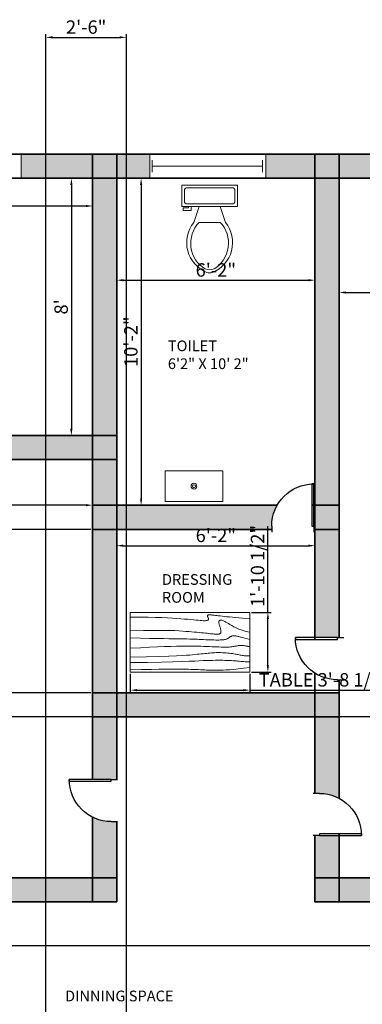
# Model space of a CAD drawing. Units: millimetres. Extents: x 2936 to 3516, y 349 to 1320.
# Tile 4 of 5: x 3187 to 3315, y 948 to 1315. Entities that reach past the tile are written whole.
import ezdxf

# ---------------------------------------------------------------- set-up
doc = ezdxf.new("R2010")
doc.units = ezdxf.units.MM
for name, color, linetype, lineweight in [('A-ANNO-DIMS', 3, 'Continuous', 13), ('A-AREA-IDEN', 190, 'Continuous', 18), ('A-FLOR-FIXT', 140, 'Continuous', 18), ('A-WALL-PATT', 50, 'Continuous', 13), ('doors', 10, 'Continuous', 25), ('furniture', 140, 'Continuous', 18), ('walls', 50, 'Continuous', 35), ('windows', 30, 'Continuous', 18)]:
    doc.layers.add(name, color=color, linetype=linetype, lineweight=lineweight)
doc.styles.get("Standard").update_dxf_attribs({"font": 'arial.ttf'})
doc.dimstyles.new('ISO-25', dxfattribs={"dimtxt": 5, "dimasz": 2.5, "dimexe": 1.25, "dimexo": 0.625, "dimtad": 1, "dimdec": 0, "dimlunit": 3, "dimtxsty": 'Standard', "dimcen": 2.5, "dimadec": 0, "dimazin": 0, "dimtfac": 1, "dimtdec": 0, "dimtmove": 0, "dimatfit": 3, "dimfxl": 1, "dimarcsym": 0})

# ---------------------------------------------------------------- blocks, each defined once
blk = doc.blocks.new('*U2')
for p, q in [((0, 0), (0, -6)), ((40, 0), (40, -6))]:
    blk.add_line(p, q)
blk.add_lwpolyline([(0, 0), (0, 40), (1.75, 40), (1.75, 0)], close=True)
blk.add_arc((0, 0), 40, 0, 90)
blk = doc.blocks.new('*U4')
for p, q in [((0, 4), (0, 0)), ((36, 4), (36, 0)), ((0, 2), (36, 2))]:
    blk.add_line(p, q)
blk = doc.blocks.new('Toilet - top')
for p, q in [((9.5, -6), (9.5, -2)), ((-10, -8.5), (-8, -8.5)), ((-10, -9.5), (-10, -8.5)), ((-7, -9.5), (-10, -9.5)), ((-8, -8.5), (-8, -8)), ((-7, -8), (-7, -9.5)), ((-4, -8), (-6, -14)), ((4, -8), (6, -14)), ((4, -14), (-4, -14))]:
    blk.add_line(p, q)
blk.add_lwpolyline([(10.5, -8), (10.5, 0), (-10.5, 0), (-10.5, -8)], close=True)
for points in [[(-9.5, -2), (-9.5, -6)], [(8.5, -1), (-8.5, -1)], [(-8.5, -7), (8.5, -7)]]:
    blk.add_lwpolyline(points)
for centre, radius, start, end in [((-8.62, -1.88), 0.884, 81.8699, 188.1301), ((8.62, -1.88), 0.884, 351.8699, 98.1301), ((-8.62, -6.12), 0.884, 171.8699, 278.1301), ((8.62, -6.12), 0.884, 261.8699, 8.1301), ((3.52, -21.58), 12.17, 141.4691, 247.9714), ((4.2, -21.82), 11.33, 136.3677, 238.9468), ((-3.52, -21.58), 12.17, 292.0284, 38.5307), ((-4.2, -21.82), 11.33, 301.053, 43.6321), ((0, -27.88), 4, 245.7318, 294.2682), ((0, -29), 4, 254.8605, 285.1395)]:
    blk.add_arc(centre, radius, start, end)
blk = doc.blocks.new('Table - Rectangular Woodgrain 60 x 30 in.')
for p, q in [((0, 0), (0, -30)), ((60, 0), (0, 0)), ((60, -30), (60, 0)), ((0, -30), (60, -30))]:
    blk.add_line(p, q)
for points in [[(0, -2.4), (4.8155, -2.418), (9.0302, -2.4688), (12.709, -2.5477), (15.9167, -2.65), (18.7181, -2.7711), (21.1781, -2.9063), (23.3616, -3.0508), (25.3333, -3.2), (27.1477, -3.3495), (28.8172, -3.4958), (30.3437, -3.636), (31.7291, -3.7667), (32.9756, -3.8849), (34.0849, -3.9875), (35.059, -4.0714), (35.9, -4.1334), (36.6114, -4.1711), (37.2041, -4.1854), (37.6906, -4.1779), (38.0833, -4.15), (38.3948, -4.1034), (38.6375, -4.0396), (38.8239, -3.9602), (38.9666, -3.8667), (39.0764, -3.7608), (39.1573, -3.6448), (39.2116, -3.521), (39.2416, -3.3917), (39.2498, -3.2593), (39.2385, -3.1261), (39.21, -2.9944), (39.1666, -2.8667), (39.111, -2.7447), (39.0468, -2.6281), (38.978, -2.5163), (38.9083, -2.4083), (38.8418, -2.3035), (38.7823, -2.201), (38.7337, -2.1001), (38.7, -2), (38.6844, -1.9003), (38.6875, -1.8021), (38.7094, -1.707), (38.75, -1.6167), (38.8094, -1.5326), (38.8875, -1.4563), (38.9844, -1.3893), (39.1, -1.3333), (39.2351, -1.2896), (39.3937, -1.2583), (39.5804, -1.2396), (39.8, -1.2333), (40.057, -1.2396), (40.3562, -1.2583), (40.7023, -1.2896), (41.1, -1.3333), (41.5547, -1.3895), (42.0755, -1.4573), (42.6721, -1.5361), (43.3542, -1.625), (44.1316, -1.7233), (45.014, -1.8302), (46.0114, -1.9449), (47.1333, -2.0667), (48.3862, -2.1947), (49.7625, -2.3281), (51.2513, -2.4663), (52.8416, -2.6083), (54.5226, -2.7535), (56.2833, -2.9011), (58.1127, -3.0501), (60, -3.2)], [(0, -9.2), (6.5759, -9.0858), (11.9385, -9.0365), (16.2527, -9.0418), (19.6833, -9.0917), (22.3952, -9.1759), (24.5531, -9.2844), (26.322, -9.4069), (27.8666, -9.5333), (29.3241, -9.6553), (30.7203, -9.7719), (32.0532, -9.8837), (33.3208, -9.9917), (34.5213, -10.0965), (35.6526, -10.199), (36.7128, -10.2999), (37.7, -10.4), (38.6129, -10.4996), (39.4531, -10.5969), (40.223, -10.6895), (40.925, -10.775), (41.5613, -10.8512), (42.1344, -10.9156), (42.6465, -10.966), (43.1, -11), (43.4976, -11.0158), (43.8437, -11.0136), (44.143, -10.9942), (44.4, -10.9583), (44.6195, -10.9069), (44.8062, -10.8406), (44.9648, -10.7603), (45.1, -10.6667), (45.2155, -10.5598), (45.3114, -10.4365), (45.3871, -10.2929), (45.4416, -10.125), (45.4743, -9.929), (45.4844, -9.7011), (45.4709, -9.4371), (45.4333, -9.1333), (45.3716, -8.7883), (45.2896, -8.4104), (45.1919, -8.0107), (45.0833, -7.6), (44.9685, -7.1893), (44.8521, -6.7896), (44.7388, -6.4117), (44.6333, -6.0667), (44.54, -5.7628), (44.4614, -5.4979), (44.4001, -5.2675), (44.3583, -5.0667), (44.3384, -4.8909), (44.3427, -4.7354), (44.3736, -4.5956), (44.4333, -4.4667), (44.5236, -4.3453), (44.6427, -4.2333), (44.7884, -4.1339), (44.9583, -4.05), (45.1501, -3.9849), (45.3614, -3.9417), (45.59, -3.9234), (45.8333, -3.9333), (46.0915, -3.9749), (46.3734, -4.0531), (46.6906, -4.1736), (47.0542, -4.3417), (47.4756, -4.5629), (47.9661, -4.8427), (48.5372, -5.1866), (49.2, -5.6), (49.9676, -6.0844), (50.8594, -6.625), (51.8965, -7.2031), (53.1, -7.8), (54.491, -8.3969), (56.0906, -8.975), (57.9199, -9.5156), (60, -10)], [(0, -12.8), (5.1847, -12.9322), (9.6213, -13.0323), (13.3963, -13.1059), (16.5958, -13.1583), (19.3063, -13.1952), (21.614, -13.2219), (23.6054, -13.2439), (25.3666, -13.2667), (26.9728, -13.2947), (28.4531, -13.3281), (29.8256, -13.3663), (31.1083, -13.4083), (32.3191, -13.4535), (33.476, -13.501), (34.597, -13.5501), (35.7, -13.6), (36.7984, -13.6497), (37.8875, -13.6979), (38.9578, -13.743), (40, -13.7833), (41.0047, -13.8174), (41.9625, -13.8438), (42.864, -13.8607), (43.7, -13.8667), (44.4631, -13.8604), (45.1552, -13.8417), (45.7801, -13.8104), (46.3416, -13.7667), (46.8439, -13.7104), (47.2906, -13.6417), (47.6858, -13.5604), (48.0333, -13.4667), (48.3375, -13.3608), (48.6042, -13.2448), (48.8396, -13.121), (49.05, -12.9917), (49.2417, -12.8593), (49.4208, -12.7261), (49.5937, -12.5944), (49.7667, -12.4667), (49.9452, -12.3451), (50.1323, -12.2313), (50.3303, -12.1268), (50.5416, -12.0333), (50.7686, -11.9524), (51.0135, -11.8854), (51.2788, -11.8341), (51.5666, -11.8), (51.8785, -11.7843), (52.2116, -11.7865), (52.562, -11.8059), (52.926, -11.8417), (53.2998, -11.8931), (53.6795, -11.9594), (54.0614, -12.0397), (54.4416, -12.1333), (54.8223, -12.2401), (55.2293, -12.3625), (55.6942, -12.5037), (56.2489, -12.6667), (56.9251, -12.8547), (57.7545, -13.0708), (58.7689, -13.3182), (60, -13.6)], [(0, -18), (5.124, -17.7273), (9.6609, -17.5057), (13.6705, -17.3303), (17.2125, -17.1958), (20.3467, -17.0973), (23.1328, -17.0297), (25.6307, -16.9878), (27.9, -16.9667), (29.9928, -16.9617), (31.9302, -16.9703), (33.7254, -16.9907), (35.3917, -17.0208), (36.9423, -17.0588), (38.3906, -17.1026), (39.7499, -17.1503), (41.0333, -17.2), (42.2519, -17.2496), (43.4073, -17.2969), (44.4986, -17.3395), (45.525, -17.375), (46.4858, -17.4012), (47.3802, -17.4156), (48.2074, -17.416), (48.9667, -17.4), (49.6583, -17.3662), (50.2872, -17.3167), (50.8595, -17.2547), (51.3812, -17.1833), (51.8584, -17.1057), (52.2971, -17.025), (52.7034, -16.9443), (53.0833, -16.8667), (53.443, -16.7951), (53.789, -16.7313), (54.128, -16.6768), (54.4666, -16.6334), (54.8115, -16.6024), (55.1693, -16.5854), (55.5465, -16.5841), (55.95, -16.6), (56.3828, -16.6337), (56.8346, -16.6823), (57.2915, -16.7418), (57.7396, -16.8084), (58.165, -16.878), (58.5539, -16.9469), (58.8924, -17.0111), (59.1666, -17.0667), (59.3679, -17.1107), (59.5078, -17.1438), (59.6032, -17.1675), (59.6708, -17.1833), (59.7275, -17.193), (59.7901, -17.1979), (59.8753, -17.1998), (60, -17.2)], [(0, -22.4), (8.0098, -22.2501), (14.4094, -22.1011), (19.4168, -21.9535), (23.25, -21.8083), (26.1269, -21.6663), (28.2656, -21.5281), (29.884, -21.3947), (31.2, -21.2667), (32.3967, -21.1448), (33.5172, -21.0292), (34.5697, -20.9198), (35.5625, -20.8167), (36.5037, -20.7198), (37.4015, -20.6292), (38.2642, -20.5448), (39.1, -20.4667), (39.9164, -20.3951), (40.7187, -20.3313), (41.5117, -20.2768), (42.3, -20.2333), (43.0883, -20.2024), (43.8812, -20.1854), (44.6836, -20.1841), (45.5, -20.2), (46.3328, -20.234), (47.1747, -20.2844), (48.0163, -20.3488), (48.8479, -20.425), (49.66, -20.5106), (50.4429, -20.6031), (51.1872, -20.7004), (51.8833, -20.8), (52.5246, -20.8999), (53.1166, -20.9995), (53.6681, -21.0983), (54.1875, -21.1958), (54.6834, -21.2919), (55.1646, -21.3859), (55.6394, -21.4777), (56.1167, -21.5667), (56.6028, -21.6515), (57.0961, -21.7266), (57.5929, -21.7852), (58.0896, -21.8208), (58.5823, -21.8268), (59.0674, -21.7964), (59.5412, -21.723), (60, -21.6)], [(0, -25.2), (8.6355, -25.0504), (15.7026, -24.9031), (21.4049, -24.7606), (25.9458, -24.625), (29.529, -24.4988), (32.3578, -24.3844), (34.6359, -24.284), (36.5667, -24.2), (38.3213, -24.1341), (39.9417, -24.0854), (41.437, -24.0523), (42.8167, -24.0333), (44.0901, -24.0268), (45.2667, -24.0313), (46.3557, -24.0451), (47.3667, -24.0667), (48.309, -24.0947), (49.1928, -24.1287), (50.0284, -24.168), (50.826, -24.2125), (51.5959, -24.2617), (52.3483, -24.3151), (53.0935, -24.3725), (53.8417, -24.4334), (54.6009, -24.497), (55.3699, -24.561), (56.1454, -24.6226), (56.9239, -24.6792), (57.7021, -24.7279), (58.4764, -24.7662), (59.2435, -24.7911), (60, -24.8)], [(0, -28.8), (5.6867, -28.6681), (10.45, -28.5698), (14.407, -28.5012), (17.675, -28.4584), (20.3711, -28.4374), (22.6125, -28.4344), (24.5164, -28.4455), (26.2, -28.4667), (27.762, -28.4947), (29.2276, -28.5281), (30.6033, -28.5663), (31.8958, -28.6084), (33.1118, -28.6535), (34.2578, -28.7011), (35.3405, -28.7501), (36.3666, -28.8), (37.3443, -28.8497), (38.288, -28.8974), (39.2137, -28.9412), (40.1375, -28.9792), (41.0753, -29.0093), (42.0432, -29.0297), (43.0572, -29.0384), (44.1333, -29.0333), (45.2936, -29.0114), (46.5843, -28.9641), (48.0579, -28.8816), (49.7666, -28.7542), (51.7629, -28.5721), (54.0989, -28.3255), (56.8272, -28.0048), (60, -27.6)]]:
    blk.add_lwpolyline(points)
blk = doc.blocks.new('*D17')
at = {"layer": 'A-ANNO-DIMS', "color": 0, "lineweight": -2, "transparency": 16777216}
for p, q in [((3205.99, 1256.28), (3207.53, 1256.28)), ((3206.28, 1253.78), (3206.28, 1162.78)), ((3205.99, 1160.28), (3207.53, 1160.28))]:
    blk.add_line(p, q, dxfattribs=at)
at = {"layer": 'A-ANNO-DIMS', "color": 0, "transparency": 16777216}
for points in [[(3205.86, 1253.78), (3206.69, 1253.78), (3206.28, 1256.28)], [(3205.86, 1162.78), (3206.69, 1162.78), (3206.28, 1160.28)]]:
    blk.add_solid(points, dxfattribs=at)
at = {"layer": 'Defpoints', "color": 0, "transparency": 16777216}
for p in [(3205.36, 1256.28), (3205.36, 1160.28), (3206.28, 1160.28)]:
    blk.add_point(p, dxfattribs=at)
at = {"layer": 'A-ANNO-DIMS', "color": 0, "transparency": 16777216, "insert": (3203.1, 1208.28), "char_height": 5, "attachment_point": 5, "rotation": 90}
blk.add_mtext("8'", dxfattribs=at)
blk = doc.blocks.new('*D18')
at = {"layer": 'A-ANNO-DIMS', "color": 0, "lineweight": -2, "transparency": 16777216}
for p, q in [((3123.19, 1246.53), (3123.19, 1247.16)), ((3211.69, 1245.91), (3125.69, 1245.91)), ((3214.19, 1246.53), (3214.19, 1247.16))]:
    blk.add_line(p, q, dxfattribs=at)
at = {"layer": 'A-ANNO-DIMS', "color": 0, "transparency": 16777216}
for points in [[(3125.69, 1246.32), (3125.69, 1245.49), (3123.19, 1245.91)], [(3211.69, 1246.32), (3211.69, 1245.49), (3214.19, 1245.91)]]:
    blk.add_solid(points, dxfattribs=at)
at = {"layer": 'Defpoints', "color": 0, "transparency": 16777216}
for p in [(3123.19, 1245.91), (3123.19, 1245.91), (3214.19, 1245.91)]:
    blk.add_point(p, dxfattribs=at)
at = {"layer": 'A-ANNO-DIMS', "color": 0, "transparency": 16777216, "insert": (3168.69, 1249.03), "char_height": 5, "attachment_point": 5}
blk.add_mtext('7\'-7"', dxfattribs=at)
blk = doc.blocks.new('*D19')
at = {"layer": 'A-ANNO-DIMS', "color": 0, "lineweight": -2, "transparency": 16777216}
for p, q in [((3231.32, 1256.28), (3233.55, 1256.28)), ((3232.3, 1253.78), (3232.3, 1136.78)), ((3231.32, 1134.28), (3233.55, 1134.28))]:
    blk.add_line(p, q, dxfattribs=at)
at = {"layer": 'A-ANNO-DIMS', "color": 0, "transparency": 16777216}
for points in [[(3231.89, 1253.78), (3232.72, 1253.78), (3232.3, 1256.28)], [(3231.89, 1136.78), (3232.72, 1136.78), (3232.3, 1134.28)]]:
    blk.add_solid(points, dxfattribs=at)
at = {"layer": 'Defpoints', "color": 0, "transparency": 16777216}
for p in [(3230.69, 1256.28), (3230.69, 1134.28), (3232.3, 1134.28)]:
    blk.add_point(p, dxfattribs=at)
at = {"layer": 'A-ANNO-DIMS', "color": 0, "transparency": 16777216, "insert": (3229.13, 1195.28), "char_height": 5, "attachment_point": 5, "rotation": 90}
blk.add_mtext('10\'-2"', dxfattribs=at)
blk = doc.blocks.new('*D20')
at = {"layer": 'A-ANNO-DIMS', "color": 0, "lineweight": -2, "transparency": 16777216}
for p, q in [((3223.19, 1218.06), (3223.19, 1216.98)), ((3225.69, 1218.23), (3294.69, 1218.23)), ((3297.19, 1218.06), (3297.19, 1216.98))]:
    blk.add_line(p, q, dxfattribs=at)
at = {"layer": 'A-ANNO-DIMS', "color": 0, "transparency": 16777216}
for points in [[(3225.69, 1218.64), (3225.69, 1217.81), (3223.19, 1218.23)], [(3294.69, 1218.64), (3294.69, 1217.81), (3297.19, 1218.23)]]:
    blk.add_solid(points, dxfattribs=at)
at = {"layer": 'Defpoints', "color": 0, "transparency": 16777216}
for p in [(3223.19, 1218.68), (3297.19, 1218.68), (3297.19, 1218.23)]:
    blk.add_point(p, dxfattribs=at)
at = {"layer": 'A-ANNO-DIMS', "color": 0, "transparency": 16777216, "insert": (3260.19, 1221.4), "char_height": 5, "attachment_point": 5}
blk.add_mtext('6\'-2"', dxfattribs=at)
blk = doc.blocks.new('*D21')
at = {"layer": 'A-ANNO-DIMS', "color": 0, "lineweight": -2, "transparency": 16777216}
for p, q in [((3306.19, 1213.25), (3306.19, 1212.4)), ((3308.69, 1213.65), (3459.69, 1213.65)), ((3462.19, 1213.25), (3462.19, 1212.4))]:
    blk.add_line(p, q, dxfattribs=at)
at = {"layer": 'A-ANNO-DIMS', "color": 0, "transparency": 16777216}
for points in [[(3308.69, 1214.07), (3308.69, 1213.23), (3306.19, 1213.65)], [(3459.69, 1214.07), (3459.69, 1213.23), (3462.19, 1213.65)]]:
    blk.add_solid(points, dxfattribs=at)
at = {"layer": 'Defpoints', "color": 0, "transparency": 16777216}
for p in [(3306.19, 1213.88), (3462.19, 1213.88), (3462.19, 1213.65)]:
    blk.add_point(p, dxfattribs=at)
at = {"layer": 'A-ANNO-DIMS', "color": 0, "transparency": 16777216, "insert": (3384.19, 1216.83), "char_height": 5, "attachment_point": 5}
blk.add_mtext("13'", dxfattribs=at)
blk = doc.blocks.new('*D24')
at = {"layer": 'A-ANNO-DIMS', "color": 0, "lineweight": -2, "transparency": 16777216}
for p, q in [((2999.19, 1134.91), (2999.19, 1135.53)), ((3214.19, 1134.91), (3214.19, 1135.53)), ((3211.69, 1134.28), (3001.69, 1134.28))]:
    blk.add_line(p, q, dxfattribs=at)
at = {"layer": 'A-ANNO-DIMS', "color": 0, "transparency": 16777216}
for points in [[(3001.69, 1134.7), (3001.69, 1133.87), (2999.19, 1134.28)], [(3211.69, 1134.7), (3211.69, 1133.87), (3214.19, 1134.28)]]:
    blk.add_solid(points, dxfattribs=at)
at = {"layer": 'Defpoints', "color": 0, "transparency": 16777216}
for p in [(2999.19, 1134.28), (2999.19, 1134.28), (3214.19, 1134.28)]:
    blk.add_point(p, dxfattribs=at)
at = {"layer": 'A-ANNO-DIMS', "color": 0, "transparency": 16777216, "insert": (3106.69, 1137.42), "char_height": 5, "attachment_point": 5}
blk.add_mtext('17\'-11"', dxfattribs=at)
blk = doc.blocks.new('*D25')
at = {"layer": 'A-ANNO-DIMS', "color": 0, "lineweight": -2, "transparency": 16777216}
for p, q in [((3223.19, 1119.81), (3223.19, 1120.43)), ((3297.19, 1119.81), (3297.19, 1120.43)), ((3225.69, 1119.18), (3294.69, 1119.18))]:
    blk.add_line(p, q, dxfattribs=at)
at = {"layer": 'A-ANNO-DIMS', "color": 0, "transparency": 16777216}
for points in [[(3225.69, 1119.6), (3225.69, 1118.76), (3223.19, 1119.18)], [(3294.69, 1119.6), (3294.69, 1118.76), (3297.19, 1119.18)]]:
    blk.add_solid(points, dxfattribs=at)
at = {"layer": 'Defpoints', "color": 0, "transparency": 16777216}
for p in [(3223.19, 1119.18), (3297.19, 1119.18), (3297.19, 1119.18)]:
    blk.add_point(p, dxfattribs=at)
at = {"layer": 'A-ANNO-DIMS', "color": 0, "transparency": 16777216, "insert": (3260.19, 1122.36), "char_height": 5, "attachment_point": 5}
blk.add_mtext('6\'-2"', dxfattribs=at)
blk = doc.blocks.new('*D53')
at = {"layer": 'A-ANNO-DIMS', "color": 0, "lineweight": -2, "transparency": 16777216}
for p, q in [((3228.24, 1071.35), (3228.24, 1064.03)), ((3272.91, 1071.35), (3272.91, 1064.03)), ((3230.74, 1065.28), (3270.41, 1065.28)), ((3272.91, 1065.28), (3325.8, 1065.28))]:
    blk.add_line(p, q, dxfattribs=at)
at = {"layer": 'A-ANNO-DIMS', "color": 0, "transparency": 16777216}
for points in [[(3230.74, 1065.69), (3230.74, 1064.86), (3228.24, 1065.28)], [(3270.41, 1065.69), (3270.41, 1064.86), (3272.91, 1065.28)]]:
    blk.add_solid(points, dxfattribs=at)
at = {"layer": 'Defpoints', "color": 0, "transparency": 16777216}
for p in [(3228.24, 1071.98), (3272.91, 1071.98), (3272.91, 1065.28)]:
    blk.add_point(p, dxfattribs=at)
at = {"layer": 'A-ANNO-DIMS', "color": 0, "transparency": 16777216, "insert": (3300.61, 1068.49), "char_height": 5, "attachment_point": 5}
blk.add_mtext('TABLE 3\'-8 1/2"', dxfattribs=at)
blk = doc.blocks.new('*D54')
at = {"layer": 'A-ANNO-DIMS', "color": 0, "lineweight": -2, "transparency": 16777216}
for p, q in [((3279.61, 1094.31), (3279.61, 1126.42)), ((3273.54, 1094.31), (3280.86, 1094.31)), ((3279.61, 1074.48), (3279.61, 1091.81)), ((3273.54, 1071.98), (3280.86, 1071.98))]:
    blk.add_line(p, q, dxfattribs=at)
at = {"layer": 'A-ANNO-DIMS', "color": 0, "transparency": 16777216}
for points in [[(3279.2, 1091.81), (3280.03, 1091.81), (3279.61, 1094.31)], [(3279.2, 1074.48), (3280.03, 1074.48), (3279.61, 1071.98)]]:
    blk.add_solid(points, dxfattribs=at)
at = {"layer": 'Defpoints', "color": 0, "transparency": 16777216}
for p in [(3272.91, 1094.31), (3279.61, 1094.31), (3272.91, 1071.98)]:
    blk.add_point(p, dxfattribs=at)
at = {"layer": 'A-ANNO-DIMS', "color": 0, "transparency": 16777216, "insert": (3276.4, 1111.61), "char_height": 5, "attachment_point": 5, "rotation": 90}
blk.add_mtext('1\'-10 1/2"', dxfattribs=at)
blk = doc.blocks.new('*D59')
at = {"layer": 'A-ANNO-DIMS', "color": 0, "lineweight": -2, "transparency": 16777216}
for p, q in [((3470.57, 1055.28), (2945.39, 1055.28)), ((2946.64, 972.36), (2946.64, 1052.78)), ((3470.57, 969.86), (2945.39, 969.86))]:
    blk.add_line(p, q, dxfattribs=at)
at = {"layer": 'A-ANNO-DIMS', "color": 0, "transparency": 16777216}
for points in [[(2946.22, 1052.78), (2947.06, 1052.78), (2946.64, 1055.28)], [(2946.22, 972.36), (2947.06, 972.36), (2946.64, 969.86)]]:
    blk.add_solid(points, dxfattribs=at)
at = {"layer": 'Defpoints', "color": 0, "transparency": 16777216}
for p in [(2946.64, 1055.28), (3471.19, 1055.28), (3471.19, 969.86)]:
    blk.add_point(p, dxfattribs=at)
at = {"layer": 'A-ANNO-DIMS', "color": 0, "transparency": 16777216, "insert": (2943.43, 1012.57), "char_height": 5, "attachment_point": 5, "rotation": 90}
blk.add_mtext('7\'-1 1/2"', dxfattribs=at)
blk = doc.blocks.new('*D65')
at = {"layer": 'A-ANNO-DIMS', "color": 0, "lineweight": -2, "transparency": 16777216}
for p, q in [((3213.57, 1125.28), (2945.39, 1125.28)), ((2946.64, 1122.78), (2946.64, 1066.78)), ((3213.57, 1064.28), (2945.39, 1064.28))]:
    blk.add_line(p, q, dxfattribs=at)
at = {"layer": 'A-ANNO-DIMS', "color": 0, "transparency": 16777216}
for points in [[(2946.22, 1122.78), (2947.06, 1122.78), (2946.64, 1125.28)], [(2946.22, 1066.78), (2947.06, 1066.78), (2946.64, 1064.28)]]:
    blk.add_solid(points, dxfattribs=at)
at = {"layer": 'Defpoints', "color": 0, "transparency": 16777216}
for p in [(3214.19, 1125.28), (2946.64, 1064.28), (3214.19, 1064.28)]:
    blk.add_point(p, dxfattribs=at)
at = {"layer": 'A-ANNO-DIMS', "color": 0, "transparency": 16777216, "insert": (2943.46, 1094.78), "char_height": 5, "attachment_point": 5, "rotation": 90}
blk.add_mtext('5\'-1"', dxfattribs=at)
blk = doc.blocks.new('*D66')
at = {"layer": 'A-ANNO-DIMS', "color": 0, "lineweight": -2, "transparency": 16777216}
for p, q in [((3196.76, 817.48), (3196.76, 1310.08)), ((3199.26, 1308.83), (3224.31, 1308.83)), ((3226.81, 817.48), (3226.81, 1310.08))]:
    blk.add_line(p, q, dxfattribs=at)
at = {"layer": 'A-ANNO-DIMS', "color": 0, "transparency": 16777216}
for points in [[(3199.26, 1309.25), (3199.26, 1308.42), (3196.76, 1308.83)], [(3224.31, 1309.25), (3224.31, 1308.42), (3226.81, 1308.83)]]:
    blk.add_solid(points, dxfattribs=at)
at = {"layer": 'Defpoints', "color": 0, "transparency": 16777216}
for p in [(3226.81, 1308.83), (3196.76, 816.86), (3226.81, 816.86)]:
    blk.add_point(p, dxfattribs=at)
at = {"layer": 'A-ANNO-DIMS', "color": 0, "transparency": 16777216, "insert": (3211.79, 1312.01), "char_height": 5, "attachment_point": 5}
blk.add_mtext('2\'-6"', dxfattribs=at)

msp = doc.modelspace()

# ---------------------------------------------------------------- hatches: boundary and pattern name
at = {"layer": 'A-WALL-PATT'}
h = msp.add_hatch(color=256, dxfattribs=at)
h.dxf.hatch_style = 1
h.paths.add_polyline_path([(2999.19, 1256.28), (2990.19, 1256.28), (2990.19, 1160.28), (2999.19, 1160.28)])
h.paths.add_polyline_path([(2999.19, 1265.28), (2990.19, 1265.28), (2990.19, 1256.28), (2999.19, 1256.28)])
h.paths.add_polyline_path([(3024.89, 1265.28), (2999.19, 1265.28), (2999.19, 1256.28), (3024.89, 1256.28)])
h.paths.add_polyline_path([(3074.24, 1160.28), (2999.19, 1160.28), (2999.19, 1151.28), (3072.14, 1151.28), (3072.14, 1152.43, -0.131652)])
h.paths.add_polyline_path([(2999.19, 1160.28), (2990.19, 1160.28), (2990.19, 1151.28), (2999.19, 1151.28)])
h.paths.add_polyline_path([(3123.19, 1256.28), (3114.19, 1256.28), (3114.19, 1160.28), (3123.19, 1160.28)])
h.paths.add_polyline_path([(3123.19, 1160.28), (3114.19, 1160.28), (3114.19, 1151.28), (3123.19, 1151.28)])
h.paths.add_polyline_path([(3114.19, 1160.28), (3087.85, 1160.28), (3087.85, 1152.43), (3087.85, 1151.28), (3114.19, 1151.28)])
h.paths.add_polyline_path([(3114.19, 1265.28), (3068.72, 1265.28), (3068.72, 1256.28), (3114.19, 1256.28)])
h.paths.add_polyline_path([(3123.19, 1265.28), (3114.19, 1265.28), (3114.19, 1256.28), (3123.19, 1256.28)])
h.paths.add_polyline_path([(3143.16, 1265.28), (3123.19, 1265.28), (3123.19, 1256.28), (3143.16, 1256.28)])
h.paths.add_polyline_path([(3214.19, 1265.28), (3187.49, 1265.28), (3187.49, 1256.28), (3214.19, 1256.28)])
h.paths.add_polyline_path([(3214.19, 1160.28), (3140.09, 1160.28, -0.121149), (3141.88, 1153), (3141.88, 1151.28), (3214.19, 1151.28)])
h.paths.add_polyline_path([(3223.19, 1256.28), (3214.19, 1256.28), (3214.19, 1160.28), (3223.19, 1160.28)])
h.paths.add_polyline_path([(3223.19, 1160.28), (3214.19, 1160.28), (3214.19, 1151.28), (3223.19, 1151.28)])
h.paths.add_polyline_path([(3223.19, 1151.28), (3214.19, 1151.28), (3214.19, 1134.28), (3223.19, 1134.28)])
h.paths.add_polyline_path([(3223.19, 1134.28), (3214.19, 1134.28), (3214.19, 1125.28), (3223.19, 1125.28)])
h.paths.add_polyline_path([(3223.19, 1125.28), (3214.19, 1125.28), (3214.19, 1064.28), (3223.19, 1064.28)])
h.paths.add_polyline_path([(3281.06, 1126.52, -0.130008), (3283.12, 1134.28), (3223.19, 1134.28), (3223.19, 1125.28), (3281.06, 1125.28)])
h.paths.add_polyline_path([(3223.19, 1265.28), (3214.19, 1265.28), (3214.19, 1256.28), (3223.19, 1256.28)])
h.paths.add_polyline_path([(3235.61, 1265.28), (3223.19, 1265.28), (3223.19, 1256.28), (3235.61, 1256.28)])
h.paths.add_polyline_path([(3297.19, 1265.28), (3278.85, 1265.28), (3278.85, 1256.28), (3297.19, 1256.28)])
h.paths.add_polyline_path([(3306.19, 1265.28), (3297.19, 1265.28), (3297.19, 1256.28), (3306.19, 1256.28)])
h.paths.add_polyline_path([(3306.19, 1256.28), (3297.19, 1256.28), (3297.19, 1134.28), (3306.19, 1134.28)])
h.paths.add_polyline_path([(3306.19, 1134.28), (3297.19, 1134.28), (3297.19, 1125.28), (3306.19, 1125.28)])
h.paths.add_polyline_path([(3306.19, 1125.28), (3297.19, 1125.28), (3297.19, 1084.87), (3305.61, 1084.87), (3306.19, 1084.87)])
h.paths.add_polyline_path([(3365.17, 1265.28), (3306.19, 1265.28), (3306.19, 1256.28), (3365.17, 1256.28)])
h.paths.add_polyline_path([(3462.19, 1265.28), (3409.24, 1265.28), (3409.24, 1256.28), (3462.19, 1256.28)])
h.paths.add_polyline_path([(3471.19, 1265.28), (3462.19, 1265.28), (3462.19, 1256.28), (3471.19, 1256.28)])
h.paths.add_polyline_path([(3471.19, 1256.28), (3462.19, 1256.28), (3462.19, 1225.41), (3471.19, 1225.41)])
h.paths.add_polyline_path([(3471.19, 1177.19), (3462.19, 1177.19), (3462.19, 1064.28), (3471.19, 1064.28)])
h.paths.add_polyline_path([(3462.19, 1064.28), (3368.33, 1064.28), (3368.33, 1055.28), (3462.19, 1055.28)])
h.paths.add_polyline_path([(3471.19, 1064.28), (3462.19, 1064.28), (3462.19, 1055.28), (3471.19, 1055.28)])
h.paths.add_polyline_path([(3471.19, 1055.28), (3462.19, 1055.28), (3462.19, 969.86), (3471.19, 969.86)])
h.paths.add_polyline_path([(3368.33, 1055.28), (3359.33, 1055.28), (3359.33, 995.28), (3368.33, 995.28)])
h.paths.add_polyline_path([(3368.33, 1064.28), (3359.33, 1064.28), (3359.33, 1055.28), (3368.33, 1055.28)])
h.paths.add_polyline_path([(3359.33, 995.28), (3306.19, 995.28), (3306.19, 986.28), (3359.33, 986.28)])
h.paths.add_polyline_path([(3368.33, 995.28), (3359.33, 995.28), (3359.33, 986.28), (3368.33, 986.28)])
h.paths.add_polyline_path([(3306.19, 995.28), (3297.19, 995.28), (3297.19, 986.28), (3306.19, 986.28)])
h.paths.add_polyline_path([(3306.19, 1011.04), (3298.85, 1011.04), (3297.19, 1011.04), (3297.19, 995.28), (3306.19, 995.28)])
h.paths.add_polyline_path([(3306.19, 1055.28), (3297.19, 1055.28), (3297.19, 1026.75), (3298.85, 1026.75, -0.122211), (3306.19, 1024.93)])
h.paths.add_polyline_path([(3306.19, 1064.28), (3297.19, 1064.28), (3297.19, 1055.28), (3306.19, 1055.28)])
h.paths.add_polyline_path([(3297.19, 1064.28), (3223.19, 1064.28), (3223.19, 1055.28), (3297.19, 1055.28)])
h.paths.add_polyline_path([(3223.19, 1064.28), (3214.19, 1064.28), (3214.19, 1055.28), (3223.19, 1055.28)])
h.paths.add_polyline_path([(3223.19, 1055.28), (3214.19, 1055.28), (3214.19, 1031.96), (3221.18, 1031.96), (3223.19, 1031.96)])
h.paths.add_polyline_path([(3223.19, 1016.25), (3221.18, 1016.25, -0.11578), (3214.19, 1017.89), (3214.19, 995.28), (3223.19, 995.28)])
h.paths.add_polyline_path([(3223.19, 995.28), (3214.19, 995.28), (3214.19, 986.28), (3223.19, 986.28)])
h.paths.add_polyline_path([(3214.19, 995.28), (3061.3, 995.28), (3061.3, 986.28), (3214.19, 986.28)])
h.paths.add_polyline_path([(2999.19, 1151.28), (2990.19, 1151.28), (2990.19, 995.28), (2999.19, 995.28)])
h.paths.add_polyline_path([(2999.19, 986.28), (2990.19, 986.28), (2990.19, 816.86), (2999.19, 816.86)])
h.paths.add_polyline_path([(2999.19, 995.28), (2990.19, 995.28), (2990.19, 986.28), (2999.19, 986.28)])
h.paths.add_polyline_path([(3016.23, 995.28), (2999.19, 995.28), (2999.19, 986.28), (3016.23, 986.28)])
h.paths.add_polyline_path([(2999.19, 807.86), (2990.19, 807.86), (2990.19, 683.86), (2999.19, 683.86)])
h.paths.add_polyline_path([(2999.19, 816.86), (2990.19, 816.86), (2990.19, 807.86), (2999.19, 807.86)])
h.paths.add_polyline_path([(3179.19, 816.86), (2999.19, 816.86), (2999.19, 807.86), (3179.19, 807.86)])
h.paths.add_polyline_path([(3188.19, 780.83), (3187.16, 780.83, -0.133677), (3179.19, 783), (3179.19, 683.86), (3188.19, 683.86)])
h.paths.add_polyline_path([(3188.19, 807.86), (3179.19, 807.86), (3179.19, 796.54), (3187.16, 796.54), (3188.19, 796.54)])
h.paths.add_polyline_path([(3188.19, 816.86), (3179.19, 816.86), (3179.19, 807.86), (3188.19, 807.86)])
h.paths.add_polyline_path([(3196.08, 816.86), (3188.19, 816.86), (3188.19, 807.86), (3196.08, 807.86)])
h.paths.add_polyline_path([(3321.19, 816.86), (3227.5, 816.86), (3227.5, 807.86), (3321.19, 807.86)])
h.paths.add_polyline_path([(3330.19, 867.56), (3321.19, 867.56), (3321.19, 816.86), (3330.19, 816.86)])
h.paths.add_polyline_path([(3330.19, 816.86), (3321.19, 816.86), (3321.19, 807.86), (3330.19, 807.86)])
h.paths.add_polyline_path([(3462.19, 816.86), (3330.19, 816.86), (3330.19, 807.86), (3462.19, 807.86)])
h.paths.add_polyline_path([(3471.19, 960.86), (3462.19, 960.86), (3462.19, 816.86), (3471.19, 816.86)])
h.paths.add_polyline_path([(3471.19, 816.86), (3462.19, 816.86), (3462.19, 807.86), (3471.19, 807.86)])
h.paths.add_polyline_path([(3471.19, 807.86), (3462.19, 807.86), (3462.19, 394.29), (3471.19, 394.29)])
h.paths.add_polyline_path([(3462.19, 715.94), (3227.5, 715.94), (3227.5, 708.13), (3227.5, 706.94), (3462.19, 706.94)])
h.paths.add_polyline_path([(3196.08, 715.94), (3188.19, 715.94), (3188.19, 706.94), (3196.08, 706.94), (3196.08, 708.13)])
h.paths.add_polyline_path([(2999.19, 674.86), (2990.19, 674.86), (2990.19, 554.86), (2999.19, 554.86)])
h.paths.add_polyline_path([(3179.19, 683.86), (2999.19, 683.86), (2999.19, 674.86), (3179.19, 674.86)])
h.paths.add_polyline_path([(2999.19, 683.86), (2990.19, 683.86), (2990.19, 674.86), (2999.19, 674.86)])
h.paths.add_polyline_path([(2999.19, 545.86), (2990.19, 545.86), (2990.19, 394.29), (2999.19, 394.29)])
h.paths.add_polyline_path([(3047.58, 554.86), (2999.19, 554.86), (2999.19, 545.86), (3047.58, 545.86)])
h.paths.add_polyline_path([(2999.19, 554.86), (2990.19, 554.86), (2990.19, 545.86), (2999.19, 545.86)])
h.paths.add_polyline_path([(3179.19, 554.86), (3096.19, 554.86), (3096.19, 545.86), (3179.19, 545.86)])
h.paths.add_polyline_path([(3188.19, 554.86), (3179.19, 554.86), (3179.19, 545.86), (3188.19, 545.86)])
h.paths.add_polyline_path([(3188.19, 652.99), (3187.11, 652.99, -0.132871), (3179.19, 655.13), (3179.19, 554.86), (3188.19, 554.86)])
h.paths.add_polyline_path([(3188.19, 683.86), (3179.19, 683.86), (3179.19, 674.86), (3188.19, 674.86)])
h.paths.add_polyline_path([(3188.19, 674.86), (3179.19, 674.86), (3179.19, 668.7), (3187.11, 668.7), (3188.19, 668.7)])
h.paths.add_polyline_path([(3462.19, 969.86), (3330.19, 969.86), (3330.19, 960.86), (3462.19, 960.86)])
h.paths.add_polyline_path([(3330.19, 969.86), (3321.19, 969.86), (3321.19, 960.86), (3330.19, 960.86)])
h.paths.add_polyline_path([(3330.19, 960.86), (3321.19, 960.86), (3321.19, 927.28), (3330.19, 927.28)])

# ---------------------------------------------------------------- linework, layer by layer
at = {"layer": 'A-FLOR-FIXT'}
msp.add_lwpolyline([(3241.23, 1135.66), (3262.84, 1135.66), (3262.84, 1147.1), (3241.23, 1147.1)], close=True, dxfattribs=at)
for radius in [1.09, 0.561]:
    msp.add_circle((3252.03, 1141.38), radius, dxfattribs=at)
at = {"layer": 'walls'}
for p, q in [((2990.19, 1265.28), (3471.19, 1265.28)), ((3214.19, 1265.28), (3214.19, 1031.96)), ((3223.19, 1265.28), (3223.19, 1031.96)), ((3297.19, 1265.28), (3297.19, 1084.19)), ((3306.19, 1265.28), (3306.19, 1084.87)), ((2990.19, 1256.28), (3471.19, 1256.28)), ((3140.09, 1160.28), (3223.19, 1160.28)), ((3141.88, 1151.28), (3223.19, 1151.28)), ((3214.19, 1134.28), (3283.12, 1134.28)), ((3296.08, 1134.28), (3306.19, 1134.28)), ((3214.19, 1125.28), (3281.06, 1125.28)), ((3296.77, 1125.28), (3306.19, 1125.28)), ((3297.19, 1071.61), (3297.19, 1026.75)), ((3306.19, 1069.16), (3306.19, 1024.93)), ((3214.19, 1064.28), (3306.19, 1064.28)), ((3214.19, 1055.28), (3306.19, 1055.28)), ((3214.19, 1017.89), (3214.19, 986.28)), ((3223.19, 1016.25), (3223.19, 986.28)), ((3297.19, 1011.04), (3297.19, 986.28)), ((3306.19, 1011.72), (3306.19, 986.28)), ((2990.19, 995.28), (3223.19, 995.28)), ((3297.19, 995.28), (3368.33, 995.28)), ((2990.19, 986.28), (3223.19, 986.28)), ((3297.19, 986.28), (3368.33, 986.28))]:
    msp.add_line(p, q, dxfattribs=at)
at = {"layer": 'windows'}
for p, q in [((3187.49, 1265.28), (3187.49, 1256.28)), ((3235.61, 1265.28), (3235.61, 1256.28)), ((3278.85, 1265.28), (3278.85, 1256.28))]:
    msp.add_line(p, q, dxfattribs=at)

# ---------------------------------------------------------------- block references
at = {"layer": 'A-FLOR-FIXT', "xscale": 0.9905491347394635, "yscale": 0.9905491347394635, "zscale": 0.9905491347394635}
msp.add_blockref('Toilet - top', (3257.88, 1253.66), dxfattribs=at)
at = {"layer": 'doors', "xscale": -0.3927729305520136, "yscale": 0.3927729305520136, "zscale": 0.3927729305520136}
msp.add_blockref('*U2', (3296.77, 1126.52), dxfattribs=at)
for p, rotation in [((3305.61, 1084.87), 90), ((3221.18, 1031.96), 90), ((3298.85, 1011.04), 270)]:
    msp.add_blockref('*U2', p, dxfattribs=dict(at, rotation=rotation))
at = {"layer": 'furniture', "xscale": 0.7445219008543091, "yscale": 0.7445219008543091, "zscale": 0.7445219008543091}
msp.add_blockref('Table - Rectangular Woodgrain 60 x 30 in.', (3228.24, 1094.31), dxfattribs=at)
at = {"layer": 'windows', "xscale": 1.142279500402185, "yscale": 1.142279500402185, "zscale": 1.142279500402185}
msp.add_blockref('*U4', (3236.47, 1258.5), dxfattribs=at)

# ---------------------------------------------------------------- texts
at = {"layer": 'A-AREA-IDEN', "char_height": 4, "attachment_point": 1}
for s, width, insert in [('TOILET\\P6\'2" X 10\' 2"', 41.0415, (3242.28, 1195.74)), ('DRESSING ROOM', 24.5933, (3240.08, 1108.57)), ('DINNING SPACE', 44.0963, (3203.92, 953.18))]:
    msp.add_mtext_dynamic_manual_height_columns(s, width=width, gutter_width=12.5, heights=[0], dxfattribs=dict(at, insert=insert))

# ---------------------------------------------------------------- dimensions: what is measured, and where the dimension line sits
at = {"layer": 'A-ANNO-DIMS'}
for base, p1, p2, override, picture, middle in [((3226.8118, 1308.8345), (3196.7646, 816.8556), (3226.8118, 816.8556), {"dimdec": 1, "dimlfac": 1, "dimrnd": 0, "dimzin": 1, "dimdsep": 46, "dimlunit": 4, "dimfrac": 2}, '*D66', (3211.7882, 1312.0124)), ((3123.19, 1245.91), (3214.19, 1245.91), (3123.19, 1245.91), {"dimclrd": 0, "dimclre": 0, "dimclrt": 0}, '*D18', (3168.69, 1249.03)), ((3297.19, 1218.23), (3223.19, 1218.68), (3297.19, 1218.68), {"dimclrd": 0, "dimclre": 0, "dimclrt": 0}, '*D20', (3260.19, 1221.4)), ((3462.19, 1213.65), (3306.19, 1213.88), (3462.19, 1213.88), {"dimclrd": 0, "dimclre": 0, "dimclrt": 0}, '*D21', (3384.19, 1216.83)), ((2999.19, 1134.28), (3214.19, 1134.28), (2999.19, 1134.28), {"dimclrd": 0, "dimclre": 0, "dimclrt": 0}, '*D24', (3106.69, 1137.42)), ((3297.19, 1119.18), (3223.19, 1119.18), (3297.19, 1119.18), {"dimclrd": 0, "dimclre": 0, "dimclrt": 0}, '*D25', (3260.19, 1122.36))]:
    dim = msp.add_linear_dim(base=base, p1=p1, p2=p2, dimstyle='ISO-25', override=override, dxfattribs=at)
    dim.commit()
    dim.dimension.update_dxf_attribs({"geometry": picture, "text_midpoint": middle})
for base, p1, p2, override, picture, middle in [((3206.28, 1160.28), (3205.36, 1256.28), (3205.36, 1160.28), {"dimclrd": 0, "dimclre": 0, "dimclrt": 0}, '*D17', (3203.1, 1208.28)), ((3232.3, 1134.28), (3230.69, 1256.28), (3230.69, 1134.28), {"dimclrd": 0, "dimclre": 0, "dimclrt": 0}, '*D19', (3229.13, 1195.28)), ((2946.64, 1064.28), (3214.19, 1125.28), (3214.19, 1064.28), {"dimdec": 1, "dimlfac": 1, "dimrnd": 0, "dimzin": 1, "dimdsep": 46, "dimlunit": 4, "dimfrac": 2}, '*D65', (2943.46, 1094.78)), ((3279.61, 1094.31), (3272.91, 1071.98), (3272.91, 1094.31), {"dimdec": 1, "dimlfac": 1, "dimrnd": 0, "dimzin": 1, "dimdsep": 46, "dimlunit": 4, "dimfrac": 2}, '*D54', (3276.4, 1111.61)), ((2946.64, 1055.28), (3471.19, 969.86), (3471.19, 1055.28), {"dimdec": 1, "dimlfac": 1, "dimrnd": 0, "dimzin": 1, "dimdsep": 46, "dimlunit": 4, "dimfrac": 2}, '*D59', (2943.43, 1012.57))]:
    dim = msp.add_linear_dim(base=base, p1=p1, p2=p2, angle=90, dimstyle='ISO-25', override=override, dxfattribs=at)
    dim.commit()
    dim.dimension.update_dxf_attribs({"geometry": picture, "text_midpoint": middle})
dim = msp.add_linear_dim(base=(3272.91, 1065.28), p1=(3228.24, 1071.98), p2=(3272.91, 1071.98), text='TABLE <>', dimstyle='ISO-25', override={"dimdec": 1, "dimlfac": 1, "dimrnd": 0, "dimzin": 1, "dimdsep": 46, "dimlunit": 4, "dimfrac": 2}, dxfattribs=at)
dim.commit()
dim.dimension.update_dxf_attribs({"geometry": '*D53', "text_midpoint": (3300.61, 1068.49)})

doc.saveas('drawing.dxf')
